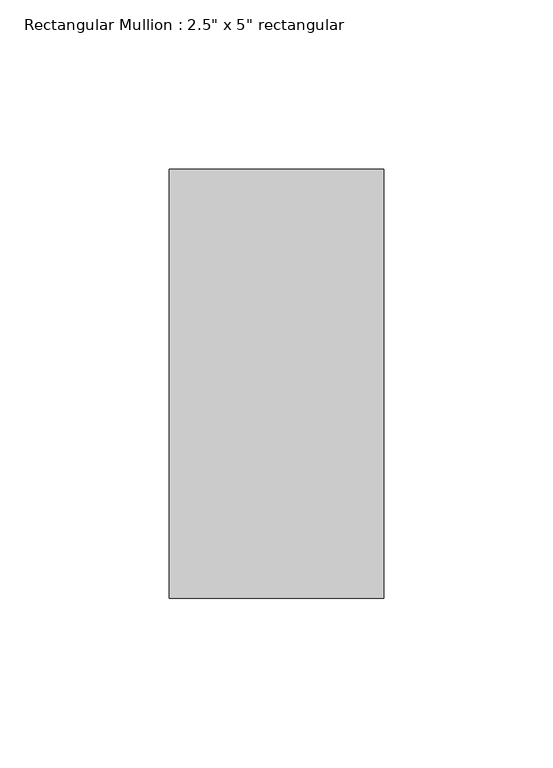
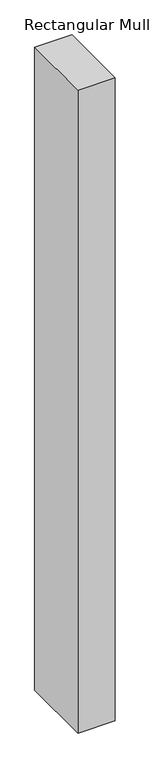
"""IFC4 building model written with IfcOpenShell, lengths in millimetres: member geometry."""

from ifc_helpers import new_model, si_unit, frame, origin, place, context, project, spatial, polyline, outline, extrude, source, transform, mapped, element, save


def member_d7472725(model_context):
    return source(origin(), model_context, "Body", "SweptSolid", [
        extrude(outline(polyline([(0.0, 63.5), (0.0, -63.5), (-63.5, -63.5), (-63.5, 63.5), (0.0, 63.5)])), frame((0.0, 0.0, -1155.7), z_axis=(0.0, 0.0, 1.0), x_axis=(1.0, 0.0, 0.0)), (0.0, 0.0, 1.0), 1155.7),
    ])


if __name__ == "__main__":
    model = new_model("IFC4")
    model_context = context("Model", 3, world=origin())
    ifc_project = project(units=[si_unit("LENGTHUNIT", "METRE", prefix="MILLI")], contexts=[model_context])
    site = spatial("IfcSite", under=ifc_project)
    building = spatial("IfcBuilding", under=site)
    placement = place(None, origin())
    member_shape = member_d7472725(model_context)
    element("IfcMember", 1, ObjectType="Rectangular Mullion : 2.5\" x 5\" rectangular", at=placement, inside=building, context=model_context, shape_type="MappedRepresentation", body=[
        mapped(member_shape, transform((0.0, 0.0, 0.0), x_axis=(1.0, 0.0, 0.0), y_axis=(0.0, 1.0, 0.0), z_axis=(0.0, 0.0, 1.0))),
    ])
    save(model, "model.ifc")

# Revit data of these elements
# Type "Rectangular Mullion : 2.5\" x 5\" rectangular"
#   built-in parameter 1007304 = 0.416667 (stored number, unit not read)
#   built-in parameter 1007301 = 0.104167 (stored number, unit not read)
#   built-in parameter 1007300 = 0.104167 (stored number, unit not read)
